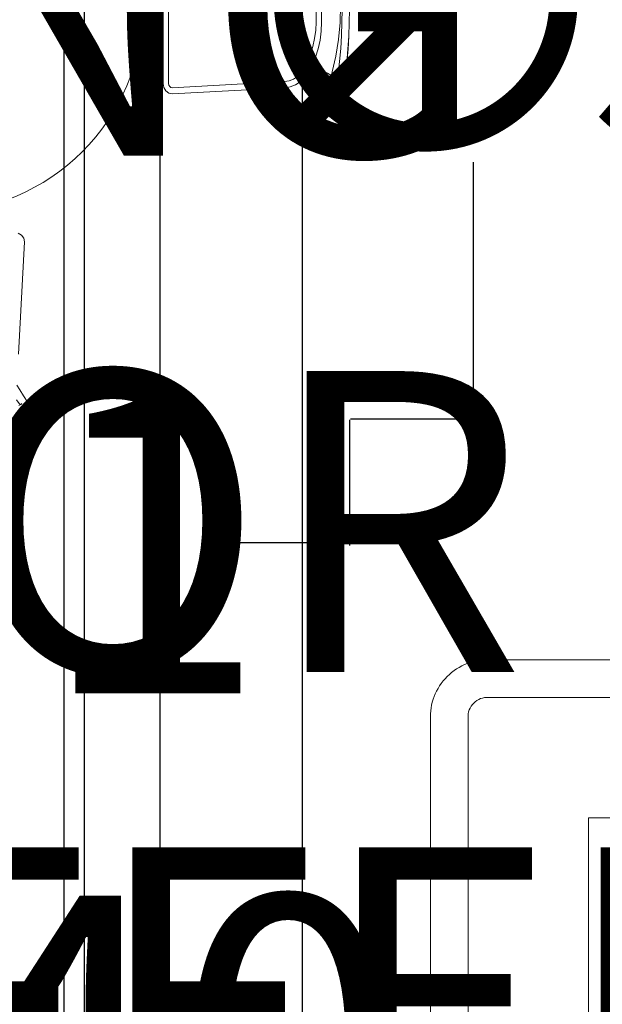
# Model space of a CAD drawing. Units: inches. Extents: x 305 to 776, y 38 to 479.
# Tile 9 of 14: x 419 to 458, y 214 to 280. Entities that reach past the tile are written whole.
import ezdxf

# ---------------------------------------------------------------- set-up
doc = ezdxf.new("R2010")
doc.units = ezdxf.units.IN
doc.header["$MEASUREMENT"] = 0
doc.layers.add('A-ANNO-DIMS', color=2, linetype='Continuous', lineweight=18)
doc.layers.add('A-FURN', color=8, linetype='Continuous', lineweight=18)
doc.styles.get("Standard").update_dxf_attribs({"font": 'arial.ttf'})
doc.dimstyles.get("Standard").update_dxf_attribs({"dimtxt": 20, "dimasz": 0.18, "dimexe": 0.18, "dimexo": 0.0625, "dimgap": 0.09, "dimtad": 0, "dimtih": 1, "dimtoh": 1, "dimdec": 4, "dimzin": 0, "dimdsep": 46, "dimtxsty": 'Standard', "dimcen": 0.09, "dimadec": 0, "dimazin": 0, "dimtfac": 1, "dimtdec": 4, "dimtofl": 0, "dimtmove": 0, "dimatfit": 3, "dimfxl": 1, "dimtolj": 1, "dimtzin": 0, "dimarcsym": 0})

# ---------------------------------------------------------------- blocks, each defined once
blk = doc.blocks.new('D')
for p, q in [((1102.721, 488.007), (1102.721, 502.387)), ((1102.722, 488.007), (1102.722, 502.387)), ((1103.227, 502.387), (1103.227, 488.007)), ((1116.749, 493.65), (1116.749, 496.744)), ((1117.254, 496.744), (1117.254, 493.65)), ((1118.955, 493.608), (1118.99, 495.197)), ((1119.121, 493.614), (1119.137, 494.821)), ((1119.809, 494.816), (1119.793, 493.593)), ((1119.794, 493.593), (1119.809, 494.816)), ((1116.709, 492.9), (1116.749, 493.65)), ((1117.254, 493.65), (1117.218, 492.825)), ((1118.808, 492.047), (1118.955, 493.608)), ((1119.076, 492.414), (1119.121, 493.614)), ((1119.793, 493.593), (1119.747, 492.372)), ((1119.748, 492.372), (1119.794, 493.593)), ((1116.45, 491.429), (1116.609, 492.158)), ((1116.609, 492.158), (1116.709, 492.9)), ((1117.218, 492.825), (1117.11, 492.009)), ((1118.559, 490.532), (1118.808, 492.047)), ((1119.002, 491.222), (1119.076, 492.414)), ((1119.747, 492.372), (1119.672, 491.16)), ((1119.673, 491.16), (1119.748, 492.372)), ((1116.234, 490.718), (1116.45, 491.429)), ((1116.932, 491.208), (1116.684, 490.43)), ((1117.11, 492.009), (1116.932, 491.208)), ((1118.9, 490.044), (1119.002, 491.222)), ((1119.672, 491.16), (1119.569, 489.961)), ((1119.569, 489.961), (1119.673, 491.16)), ((1115.961, 490.033), (1116.234, 490.718)), ((1116.684, 490.43), (1116.37, 489.684)), ((1118.235, 489.103), (1118.559, 490.532)), ((1115.367, 488.998), (1115.635, 489.378)), ((1115.635, 489.378), (1115.961, 490.033)), ((1116.37, 489.684), (1116.01, 488.971)), ((1116.582, 489.267), (1116.658, 489.358)), ((1116.658, 489.358), (1116.758, 489.415)), ((1116.758, 489.415), (1116.869, 489.432)), ((1116.869, 489.432), (1117.193, 489.288)), ((1118.773, 488.882), (1118.9, 490.044)), ((1119.569, 489.961), (1119.44, 488.783)), ((1119.44, 488.783), (1119.569, 489.961)), ((1114.274, 488.266), (1114.679, 488.428)), ((1114.679, 488.428), (1115.048, 488.675)), ((1115.048, 488.675), (1115.367, 488.998)), ((1115.673, 488.537), (1115.288, 488.171)), ((1115.674, 488.537), (1115.289, 488.171)), ((1115.814, 488.719), (1115.673, 488.537)), ((1116.01, 488.971), (1115.674, 488.537)), ((1115.848, 488.69), (1115.814, 488.719)), ((1115.838, 488.606), (1115.87, 488.761)), ((1115.838, 488.61), (1115.848, 488.69)), ((1115.84, 488.529), (1115.838, 488.61)), ((1115.858, 488.449), (1115.838, 488.606)), ((1115.857, 488.45), (1115.84, 488.529)), ((1115.885, 488.376), (1115.857, 488.45)), ((1115.927, 488.31), (1115.858, 488.449)), ((1115.87, 488.761), (1115.949, 488.893)), ((1115.949, 488.893), (1116.065, 488.984)), ((1116.065, 488.984), (1116.202, 489.022)), ((1116.202, 489.022), (1116.342, 489.002)), ((1116.342, 489.002), (1116.467, 488.926)), ((1116.661, 488.761), (1116.467, 488.926)), ((1116.527, 489.027), (1116.536, 489.152)), ((1116.556, 488.905), (1116.527, 489.027)), ((1116.536, 489.152), (1116.582, 489.267)), ((1116.619, 488.802), (1116.556, 488.905)), ((1116.71, 488.728), (1116.619, 488.802)), ((1116.882, 488.62), (1116.71, 488.728)), ((1116.882, 488.62), (1116.912, 488.601)), ((1116.912, 488.601), (1117.177, 488.459)), ((1117.177, 488.459), (1117.495, 488.282)), ((1117.193, 489.288), (1117.471, 489.14)), ((1117.471, 489.14), (1117.796, 488.959)), ((1117.796, 488.959), (1118.097, 488.784)), ((1117.999, 488.732), (1118.067, 488.754)), ((1118.067, 488.754), (1118.085, 488.769)), ((1118.085, 488.769), (1118.126, 488.824)), ((1118.126, 488.824), (1118.176, 488.94)), ((1118.176, 488.94), (1118.235, 489.103)), ((1118.55, 488.219), (1118.695, 488.416)), ((1118.633, 487.766), (1118.773, 488.882)), ((1118.695, 488.416), (1118.722, 488.478)), ((1119.44, 488.783), (1119.291, 487.602)), ((1119.292, 487.602), (1119.44, 488.783)), ((1102.785, 487.645), (1102.721, 488.007)), ((1102.786, 487.645), (1102.722, 488.007)), ((1102.968, 487.338), (1102.785, 487.645)), ((1102.968, 487.338), (1102.786, 487.645)), ((1103.227, 488.007), (1103.252, 487.863)), ((1103.252, 487.863), (1103.325, 487.74)), ((1103.325, 487.74), (1103.434, 487.658)), ((1103.434, 487.658), (1103.563, 487.629)), ((1113.874, 487.629), (1103.562, 487.061)), ((1103.563, 487.629), (1113.85, 488.196)), ((1113.874, 487.629), (1103.563, 487.061)), ((1113.85, 488.196), (1114.274, 488.266)), ((1114.372, 487.709), (1113.874, 487.629)), ((1114.373, 487.709), (1113.874, 487.629)), ((1114.849, 487.892), (1114.372, 487.709)), ((1114.85, 487.892), (1114.373, 487.709)), ((1115.288, 488.171), (1114.849, 487.892)), ((1115.289, 488.171), (1114.85, 487.892)), ((1115.926, 488.31), (1115.885, 488.376)), ((1116.718, 487.771), (1115.926, 488.31)), ((1115.927, 488.31), (1116.719, 487.771)), ((1117.144, 487.504), (1116.718, 487.771)), ((1116.719, 487.771), (1117.145, 487.504)), ((1117.406, 488.332), (1117.556, 488.212)), ((1117.495, 488.282), (1117.914, 488.047)), ((1117.556, 488.212), (1118.069, 487.816)), ((1117.914, 488.047), (1118.139, 488.006)), ((1118.069, 487.816), (1118.536, 487.468)), ((1118.255, 488.039), (1118.139, 488.006)), ((1118.255, 488.039), (1118.371, 488.076)), ((1118.371, 488.076), (1118.55, 488.219)), ((1118.534, 487.462), (1118.585, 487.596)), ((1118.585, 487.596), (1118.633, 487.766)), ((1119.291, 487.602), (1119.217, 487.335)), ((1119.217, 487.335), (1119.292, 487.602)), ((1103.241, 487.133), (1102.968, 487.338)), ((1103.241, 487.133), (1102.968, 487.338)), ((1103.562, 487.061), (1103.241, 487.133)), ((1103.563, 487.061), (1103.241, 487.133)), ((1117.691, 487.151), (1117.144, 487.504)), ((1117.145, 487.504), (1117.692, 487.151)), ((1118.3, 486.754), (1117.691, 487.151)), ((1117.692, 487.151), (1118.301, 486.754)), ((1118.348, 486.715), (1118.3, 486.754)), ((1118.349, 486.715), (1118.301, 486.754)), ((1118.455, 486.681), (1118.348, 486.715)), ((1118.349, 486.715), (1118.455, 486.681)), ((1118.407, 487.302), (1118.495, 487.394)), ((1118.575, 486.653), (1118.455, 486.681)), ((1118.576, 486.653), (1118.455, 486.681)), ((1118.495, 487.394), (1118.534, 487.462)), ((1118.703, 486.689), (1118.575, 486.653)), ((1118.576, 486.653), (1118.704, 486.688)), ((1118.83, 486.733), (1118.703, 486.689)), ((1118.704, 486.688), (1118.831, 486.733)), ((1119.007, 486.901), (1118.83, 486.733)), ((1118.831, 486.733), (1119.008, 486.901)), ((1119.129, 487.107), (1119.007, 486.901)), ((1119.008, 486.901), (1119.13, 487.107)), ((1119.217, 487.335), (1119.129, 487.107)), ((1119.13, 487.107), (1119.217, 487.335)), ((1089.743, 474.114), (1089.436, 474.296)), ((1089.743, 474.113), (1089.436, 474.295)), ((1089.948, 473.841), (1089.743, 474.114)), ((1089.948, 473.84), (1089.743, 474.113)), ((1089.453, 463.208), (1090.02, 473.519)), ((1089.453, 463.207), (1090.02, 473.518)), ((1090.02, 473.519), (1089.948, 473.841)), ((1090.02, 473.518), (1089.948, 473.84)), ((1089.577, 459.938), (1089.31, 460.363)), ((1089.31, 460.363), (1089.577, 459.937)), ((1089.93, 459.39), (1089.577, 459.938)), ((1089.577, 459.937), (1089.93, 459.39)), ((1089.265, 459.012), (1089.614, 458.545)), ((1089.779, 458.675), (1089.687, 458.587)), ((1090.328, 458.781), (1089.93, 459.39)), ((1089.93, 459.39), (1090.328, 458.78)), ((1090.367, 458.733), (1090.328, 458.781)), ((1090.367, 458.732), (1090.328, 458.78)), ((1090.4, 458.627), (1090.367, 458.733)), ((1090.367, 458.732), (1090.4, 458.626)), ((1090.428, 458.506), (1090.4, 458.627)), ((1090.428, 458.506), (1090.4, 458.626)), ((1089.48, 457.791), (1089.746, 457.865)), ((1089.746, 457.864), (1089.48, 457.79)), ((1089.62, 458.547), (1089.485, 458.496)), ((1089.687, 458.587), (1089.62, 458.547)), ((1089.746, 457.865), (1089.975, 457.953)), ((1089.975, 457.952), (1089.746, 457.864)), ((1089.975, 457.953), (1090.18, 458.075)), ((1090.18, 458.074), (1089.975, 457.952)), ((1090.18, 458.075), (1090.348, 458.251)), ((1090.348, 458.25), (1090.18, 458.074)), ((1090.348, 458.251), (1090.393, 458.379)), ((1090.393, 458.378), (1090.348, 458.25)), ((1090.393, 458.379), (1090.428, 458.506)), ((1090.428, 458.506), (1090.393, 458.378))]:
    blk.add_line(p, q)
blk.add_circle((1081.884, 495.197), 18.987)
blk = doc.blocks.new('carp')
for p, q in [((853.971, 318.32), (853.971, 318.33)), ((857.971, 314.33), (857.965, 314.33))]:
    blk.add_line(p, q)
for points in [[(853.971, 318.33), (831.574, 318.33)], [(853.971, 315.83), (831.574, 315.83)], [(827.971, 314.727), (827.971, 277.33)], [(830.471, 314.727), (830.471, 277.33)], [(855.471, 277.33), (855.471, 314.33)], [(857.971, 277.33), (857.971, 314.33)], [(831.971, 275.83), (853.971, 275.83)], [(831.971, 273.33), (853.971, 273.33)]]:
    blk.add_lwpolyline(points)
blk.add_lwpolyline([(838.471, 307.83), (838.471, 283.83), (847.471, 283.83), (847.471, 307.83)], close=True)
for centre, radius, start, end in [((831.772, 314.528), 3.807, 87.01121, 182.98879), ((853.855, 314.211), 4.111, 358.88612, 88.46258), ((831.772, 314.528), 1.307, 87.01121, 182.98879), ((853.855, 314.211), 1.611, 358.88612, 88.46258), ((832.523, 277.882), 2.086, 186.91602, 263.08398), ((853.419, 277.882), 2.086, 276.91602, 353.08398), ((832.523, 277.882), 4.586, 186.91602, 263.08398), ((853.419, 277.882), 4.586, 276.91602, 353.08398)]:
    blk.add_arc(centre, radius, start, end)
blk = doc.blocks.new('*D19')
at = {"layer": 'A-ANNO-DIMS', "color": 0, "lineweight": -2, "transparency": 16777216}
for p, q in [((557.633, 250.82), (557.633, 245.977)), ((589.133, 250.82), (589.133, 245.977)), ((557.633, 246.157), (557.453, 246.157)), ((588.953, 246.157), (557.813, 246.157))]:
    blk.add_line(p, q, dxfattribs=at)
at = {"layer": 'A-ANNO-DIMS', "color": 0, "transparency": 16777216}
for points in [[(557.813, 246.187), (557.813, 246.127), (557.633, 246.157)], [(588.953, 246.187), (588.953, 246.127), (589.133, 246.157)]]:
    blk.add_solid(points, dxfattribs=at)
at = {"layer": 'Defpoints', "color": 0, "transparency": 16777216}
for p in [(557.633, 250.882), (589.133, 250.882), (557.633, 246.157)]:
    blk.add_point(p, dxfattribs=at)
at = {"layer": 'A-ANNO-DIMS', "color": 0, "transparency": 16777216, "insert": (463.393, 246.157), "char_height": 20, "attachment_point": 5}
blk.add_mtext('\\A1;DOOR 32 TYP.', dxfattribs=at)
blk = doc.blocks.new('*D33')
at = {"layer": 'A-ANNO-DIMS', "color": 0, "lineweight": -2, "transparency": 16777216}
for p, q in [((440.927, 307.949), (449.29, 307.949)), ((449.11, 307.769), (449.11, 290.896)), ((449.11, 253.161), (449.11, 270.034)), ((440.927, 252.981), (449.29, 252.981))]:
    blk.add_line(p, q, dxfattribs=at)
at = {"layer": 'A-ANNO-DIMS', "color": 0, "transparency": 16777216}
for points in [[(449.08, 307.769), (449.14, 307.769), (449.11, 307.949)], [(449.08, 253.161), (449.14, 253.161), (449.11, 252.981)]]:
    blk.add_solid(points, dxfattribs=at)
at = {"layer": 'Defpoints', "color": 0, "transparency": 16777216}
for p in [(440.864, 307.949), (449.11, 307.949), (440.864, 252.981)]:
    blk.add_point(p, dxfattribs=at)
at = {"layer": 'A-ANNO-DIMS', "color": 0, "transparency": 16777216, "insert": (449.11, 280.465), "char_height": 20, "attachment_point": 5}
blk.add_mtext('\\A1;DINING SET 55', dxfattribs=at)
blk = doc.blocks.new('*D34')
at = {"layer": 'A-ANNO-DIMS', "color": 0, "lineweight": -2, "transparency": 16777216}
for p, q in [((399.621, 252.919), (399.621, 244.556)), ((440.864, 252.919), (440.864, 244.556)), ((399.801, 244.736), (407.356, 244.736)), ((440.684, 244.736), (433.129, 244.736))]:
    blk.add_line(p, q, dxfattribs=at)
at = {"layer": 'A-ANNO-DIMS', "color": 0, "transparency": 16777216}
for points in [[(399.801, 244.766), (399.801, 244.706), (399.621, 244.736)], [(440.684, 244.766), (440.684, 244.706), (440.864, 244.736)]]:
    blk.add_solid(points, dxfattribs=at)
at = {"layer": 'Defpoints', "color": 0, "transparency": 16777216}
for p in [(399.621, 252.981), (440.864, 252.981), (440.864, 244.736)]:
    blk.add_point(p, dxfattribs=at)
at = {"layer": 'A-ANNO-DIMS', "color": 0, "transparency": 16777216, "insert": (420.242, 244.736), "char_height": 20, "attachment_point": 5}
blk.add_mtext('\\A1;41', dxfattribs=at)
blk = doc.blocks.new('*D37')
at = {"layer": 'A-ANNO-DIMS', "color": 0, "lineweight": -2, "transparency": 16777216}
for p, q in [((476.346, 237.029), (483.222, 237.029)), ((483.042, 236.849), (483.042, 224.939)), ((483.042, 192.153), (483.042, 204.063)), ((476.346, 191.973), (483.222, 191.973))]:
    blk.add_line(p, q, dxfattribs=at)
at = {"layer": 'A-ANNO-DIMS', "color": 0, "transparency": 16777216}
for points in [[(483.012, 236.849), (483.072, 236.849), (483.042, 237.029)], [(483.012, 192.153), (483.072, 192.153), (483.042, 191.973)]]:
    blk.add_solid(points, dxfattribs=at)
at = {"layer": 'Defpoints', "color": 0, "transparency": 16777216}
for p in [(476.283, 237.029), (483.042, 237.029), (476.283, 191.973)]:
    blk.add_point(p, dxfattribs=at)
at = {"layer": 'A-ANNO-DIMS', "color": 0, "transparency": 16777216, "insert": (483.042, 214.501), "char_height": 20, "attachment_point": 5}
blk.add_mtext('\\A1;COFFEE TABLE 45', dxfattribs=at)
blk = doc.blocks.new('*D39')
at = {"layer": 'A-ANNO-DIMS', "color": 0, "lineweight": -2, "transparency": 16777216}
for p, q in [((404.195, 231.292), (410.313, 231.292)), ((410.133, 231.112), (410.133, 221.593)), ((410.133, 191.472), (410.133, 200.99)), ((404.195, 191.292), (410.313, 191.292))]:
    blk.add_line(p, q, dxfattribs=at)
at = {"layer": 'A-ANNO-DIMS', "color": 0, "transparency": 16777216}
for points in [[(410.103, 231.112), (410.163, 231.112), (410.133, 231.292)], [(410.103, 191.472), (410.163, 191.472), (410.133, 191.292)]]:
    blk.add_solid(points, dxfattribs=at)
at = {"layer": 'Defpoints', "color": 0, "transparency": 16777216}
for p in [(404.133, 231.292), (410.133, 231.292), (404.133, 191.292)]:
    blk.add_point(p, dxfattribs=at)
at = {"layer": 'A-ANNO-DIMS', "color": 0, "transparency": 16777216, "insert": (410.133, 211.292), "char_height": 20, "attachment_point": 5}
blk.add_mtext('\\A1;TV 40', dxfattribs=at)
blk = doc.blocks.new('*D60')
at = {"layer": 'A-ANNO-DIMS', "color": 0, "lineweight": -2, "transparency": 16777216}
for p, q in [((428.263, 331.82), (428.263, 51.201)), ((465.633, 331.82), (465.633, 51.201)), ((428.443, 51.381), (465.453, 51.381)), ((465.633, 51.381), (465.813, 51.381))]:
    blk.add_line(p, q, dxfattribs=at)
at = {"layer": 'A-ANNO-DIMS', "color": 0, "transparency": 16777216}
for points in [[(428.443, 51.411), (428.443, 51.351), (428.263, 51.381)], [(465.453, 51.411), (465.453, 51.351), (465.633, 51.381)]]:
    blk.add_solid(points, dxfattribs=at)
at = {"layer": 'Defpoints', "color": 0, "transparency": 16777216}
for p in [(428.263, 331.882), (465.633, 331.882), (465.633, 51.381)]:
    blk.add_point(p, dxfattribs=at)
at = {"layer": 'A-ANNO-DIMS', "color": 0, "transparency": 16777216, "insert": (499.641, 51.381), "char_height": 20, "attachment_point": 5}
blk.add_mtext('\\A1;37.37', dxfattribs=at)
blk = doc.blocks.new('*D61')
at = {"layer": 'A-ANNO-DIMS', "color": 0, "lineweight": -2, "transparency": 16777216}
for p, q in [((437.73, 398.686), (437.73, 51.201)), ((465.633, 398.686), (465.633, 51.201)), ((437.91, 51.381), (465.453, 51.381)), ((465.633, 51.381), (465.813, 51.381))]:
    blk.add_line(p, q, dxfattribs=at)
at = {"layer": 'A-ANNO-DIMS', "color": 0, "transparency": 16777216}
for points in [[(437.91, 51.411), (437.91, 51.351), (437.73, 51.381)], [(465.453, 51.411), (465.453, 51.351), (465.633, 51.381)]]:
    blk.add_solid(points, dxfattribs=at)
at = {"layer": 'Defpoints', "color": 0, "transparency": 16777216}
for p in [(437.73, 398.749), (465.633, 398.749), (465.633, 51.381)]:
    blk.add_point(p, dxfattribs=at)
at = {"layer": 'A-ANNO-DIMS', "color": 0, "transparency": 16777216, "insert": (492.069, 51.381), "char_height": 20, "attachment_point": 5}
blk.add_mtext('\\A1;27.9', dxfattribs=at)
blk = doc.blocks.new('*D62')
at = {"layer": 'A-ANNO-DIMS', "color": 0, "lineweight": -2, "transparency": 16777216}
for p, q in [((399.633, 336.32), (399.633, 51.201)), ((423.233, 336.32), (423.233, 51.201)), ((399.813, 51.381), (423.053, 51.381)), ((423.233, 51.381), (423.413, 51.381))]:
    blk.add_line(p, q, dxfattribs=at)
at = {"layer": 'A-ANNO-DIMS', "color": 0, "transparency": 16777216}
for points in [[(399.813, 51.411), (399.813, 51.351), (399.633, 51.381)], [(423.053, 51.411), (423.053, 51.351), (423.233, 51.381)]]:
    blk.add_solid(points, dxfattribs=at)
at = {"layer": 'Defpoints', "color": 0, "transparency": 16777216}
for p in [(399.633, 336.382), (423.233, 336.382), (423.233, 51.381)]:
    blk.add_point(p, dxfattribs=at)
at = {"layer": 'A-ANNO-DIMS', "color": 0, "transparency": 16777216, "insert": (449.642, 51.381), "char_height": 20, "attachment_point": 5}
blk.add_mtext('\\A1;23.6', dxfattribs=at)
blk = doc.blocks.new('*D65')
at = {"layer": 'A-ANNO-DIMS', "color": 0, "lineweight": -2, "transparency": 16777216}
for p, q in [((399.633, 351.219), (399.633, 51.201)), ((421.89, 351.219), (421.89, 51.201)), ((399.813, 51.381), (421.71, 51.381)), ((421.89, 51.381), (422.07, 51.381))]:
    blk.add_line(p, q, dxfattribs=at)
at = {"layer": 'A-ANNO-DIMS', "color": 0, "transparency": 16777216}
for points in [[(399.813, 51.411), (399.813, 51.351), (399.633, 51.381)], [(421.71, 51.411), (421.71, 51.351), (421.89, 51.381)]]:
    blk.add_solid(points, dxfattribs=at)
at = {"layer": 'Defpoints', "color": 0, "transparency": 16777216}
for p in [(399.633, 351.281), (421.89, 351.281), (421.89, 51.381)]:
    blk.add_point(p, dxfattribs=at)
at = {"layer": 'A-ANNO-DIMS', "color": 0, "transparency": 16777216, "insert": (463.844, 51.381), "char_height": 20, "attachment_point": 5}
blk.add_mtext('\\A1;22.257', dxfattribs=at)
blk = doc.blocks.new('*D75')
at = {"layer": 'A-ANNO-DIMS', "color": 0, "lineweight": -2, "transparency": 16777216}
for p, q in [((413.291, 280.465), (413.471, 280.465)), ((413.381, 280.375), (413.381, 280.555)), ((435.396, 280.465), (427.32, 280.465))]:
    blk.add_line(p, q, dxfattribs=at)
at = {"layer": 'A-ANNO-DIMS', "color": 0, "transparency": 16777216}
blk.add_solid([(427.32, 280.495), (427.32, 280.435), (427.14, 280.465)], dxfattribs=at)
at = {"layer": 'Defpoints', "color": 0, "transparency": 16777216}
for p in [(399.621, 280.466), (427.14, 280.465)]:
    blk.add_point(p, dxfattribs=at)
at = {"layer": 'A-ANNO-DIMS', "color": 0, "transparency": 16777216, "insert": (480.009, 280.465), "char_height": 20, "attachment_point": 5}
blk.add_mtext('\\A1;∅27.52', dxfattribs=at)

msp = doc.modelspace()

# ---------------------------------------------------------------- block references
at = {"layer": 'A-FURN', "xscale": 0.724692399516523, "yscale": 0.724692399516523, "zscale": 0.724692399516523}
msp.add_blockref('D', (-370.653, -78.4001), dxfattribs=at)
at = {"layer": 'A-FURN'}
msp.add_blockref('carp', (-381.7264, -81.357), dxfattribs=at)

# ---------------------------------------------------------------- dimensions: what is measured, and where the dimension line sits
at = {"layer": 'A-ANNO-DIMS'}
for base, p1, p2, override, picture, middle in [((465.6329, 51.3805), (437.7303, 398.7487), (465.6329, 398.7487), {"dimdec": 1, "dimlfac": 1, "dimrnd": 0, "dimzin": 0, "dimdsep": 46, "dimlunit": 2}, '*D61', (492.0693, 51.3805)), ((421.8895, 51.3805), (399.6329, 351.2815), (421.8895, 351.2815), {"dimdec": 3, "dimlfac": 1, "dimrnd": 0, "dimzin": 0, "dimdsep": 46, "dimlunit": 2}, '*D65', (463.8444, 51.3805)), ((423.2329, 51.3805), (399.6329, 336.382), (423.2329, 336.382), {"dimdec": 1, "dimlfac": 1, "dimrnd": 0, "dimzin": 0, "dimdsep": 46, "dimlunit": 2}, '*D62', (449.6421, 51.3805)), ((465.6329, 51.3805), (428.2629, 331.882), (465.6329, 331.882), {"dimdec": 2, "dimlfac": 1, "dimrnd": 0, "dimzin": 0, "dimdsep": 46, "dimlunit": 2}, '*D60', (499.641, 51.3805)), ((440.8644, 244.7363), (399.6205, 252.9815), (440.8644, 252.9815), {"dimdec": 0, "dimlfac": 1, "dimrnd": 0, "dimzin": 0, "dimdsep": 46, "dimlunit": 2}, '*D34', (420.2425, 244.7363))]:
    dim = msp.add_linear_dim(base=base, p1=p1, p2=p2, dimstyle='Standard', override=override, dxfattribs=at)
    dim.commit()
    dim.dimension.update_dxf_attribs({"geometry": picture, "text_midpoint": middle})
for base, p1, p2, angle, text, picture, middle in [((449.1096, 307.9493), (440.8644, 252.9815), (440.8644, 307.9493), 90, 'DINING SET <>', '*D33', (449.1096, 280.4654)), ((557.6329062952, 246.15704135), (589.1329062952, 250.88204135), (557.6329062952, 250.88204135), 180, 'DOOR <> TYP.', '*D19', (463.3929199378, 246.15704135)), ((483.0416, 237.0288), (476.2832, 191.9726), (476.2832, 237.0288), 90, 'COFFEE TABLE <>', '*D37', (483.0416, 214.5007)), ((410.1329, 231.2915), (404.1329, 191.2915), (404.1329, 231.2915), 90, 'TV <>', '*D39', (410.1329, 211.2915))]:
    dim = msp.add_linear_dim(base=base, p1=p1, p2=p2, angle=angle, text=text, dimstyle='Standard', override={"dimdec": 0, "dimlfac": 1, "dimrnd": 0, "dimzin": 0, "dimdsep": 46, "dimlunit": 2}, dxfattribs=at)
    dim.commit()
    dim.dimension.update_dxf_attribs({"geometry": picture, "text_midpoint": middle})
dim = msp.add_diameter_dim_2p(p1=(399.6205, 280.4658), p2=(427.1405, 280.465), dimstyle='Standard', override={"dimdec": 2, "dimlfac": 1, "dimrnd": 0, "dimzin": 0, "dimdsep": 46, "dimlunit": 2}, dxfattribs=at)
dim.commit()
dim.dimension.update_dxf_attribs({"geometry": '*D75', "text_midpoint": (435.3965, 280.4648), "dimtype": 163})

doc.saveas('drawing.dxf')
